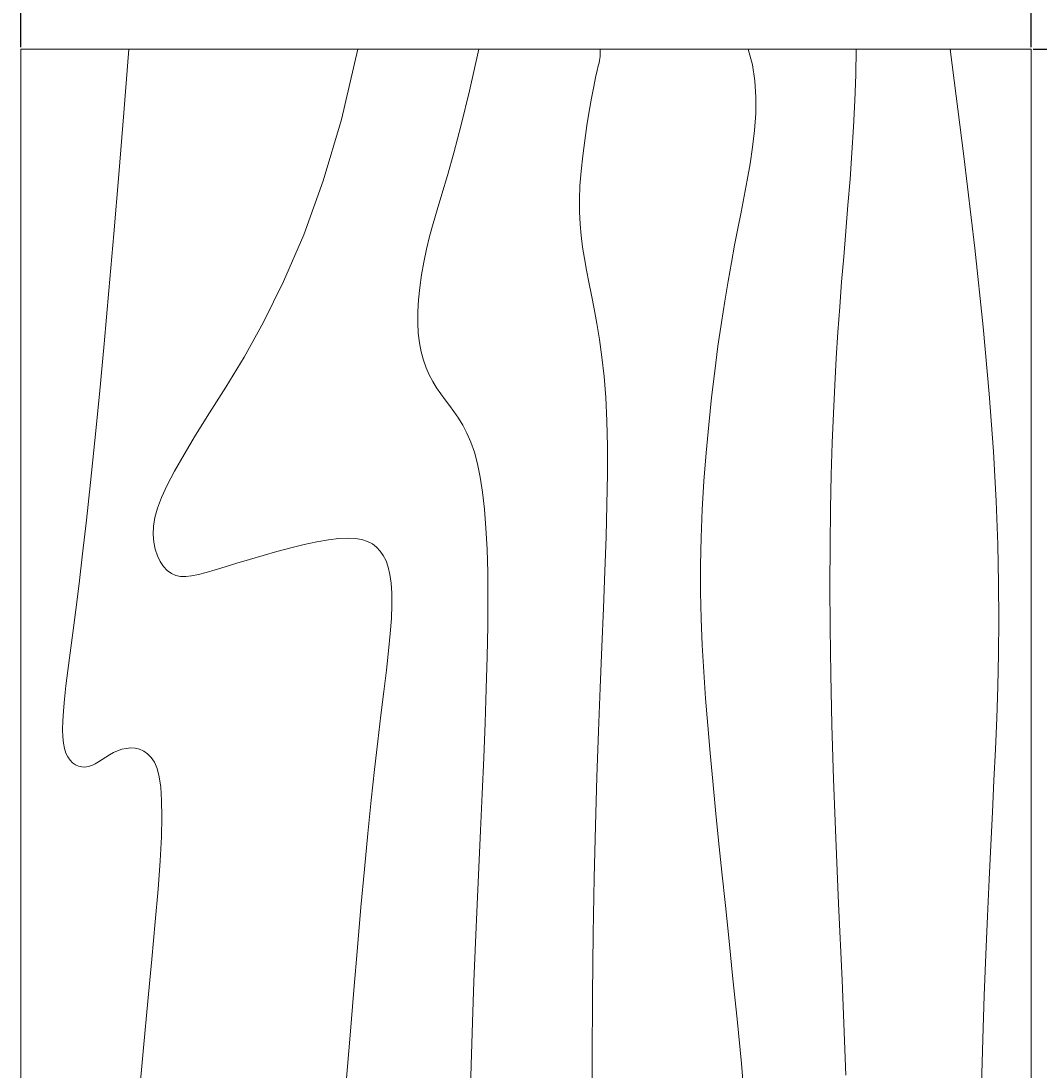
# Model space of a CAD drawing. Units: inches. Extents: x -105 to 1196, y -792 to 119.
# Tile 13 of 23: x 232 to 262, y -349 to -318. Entities that reach past the tile are written whole.
import ezdxf

# ---------------------------------------------------------------- set-up
doc = ezdxf.new("R2010")
doc.units = ezdxf.units.IN
doc.header["$MEASUREMENT"] = 0
doc.layers.add('A-ANNO-DIMS', color=2, linetype='Continuous', lineweight=18)
doc.layers.add('A-FURN', color=8, linetype='Continuous', lineweight=18)
doc.styles.get("Standard").update_dxf_attribs({"font": 'arial.ttf'})
doc.dimstyles.get("Standard").update_dxf_attribs({"dimtxt": 0.18, "dimasz": 0.18, "dimexe": 0.18, "dimexo": 0.0625, "dimgap": 0.09, "dimtad": 0, "dimtih": 1, "dimtoh": 1, "dimdec": 1, "dimzin": 0, "dimdsep": 46, "dimlunit": 4, "dimtxsty": 'Standard', "dimcen": 0.09, "dimadec": 0, "dimazin": 0, "dimtfac": 1, "dimtdec": 1, "dimtofl": 0, "dimtmove": 0, "dimatfit": 3, "dimfxl": 1, "dimtolj": 1, "dimtzin": 0, "dimarcsym": 0})

# ---------------------------------------------------------------- blocks, each defined once
blk = doc.blocks.new('Table - Rectangular Woodgrain 60 x 30 in.')
for p, q in [((60, 0), (0, 0)), ((60, -30), (60, 0)), ((0, -30), (60, -30))]:
    blk.add_line(p, q)
for points in [[(28.8172, -3.4958), (30.3437, -3.636), (31.7291, -3.7667), (32.9756, -3.8849), (34.0849, -3.9875), (35.059, -4.0714), (35.9, -4.1334), (36.6114, -4.1711), (37.2041, -4.1854), (37.6906, -4.1779), (38.0833, -4.15), (38.3948, -4.1034), (38.6375, -4.0396), (38.8239, -3.9602), (38.9666, -3.8667), (39.0764, -3.7608), (39.1573, -3.6448), (39.2116, -3.521), (39.2416, -3.3917), (39.2498, -3.2593), (39.2385, -3.1261), (39.21, -2.9944), (39.1666, -2.8667), (39.111, -2.7447), (39.0468, -2.6281), (38.978, -2.5163), (38.9083, -2.4083), (38.8418, -2.3035), (38.7823, -2.201), (38.7337, -2.1001), (38.7, -2), (38.6844, -1.9003), (38.6875, -1.8021), (38.7094, -1.707), (38.75, -1.6167), (38.8094, -1.5326), (38.8875, -1.4563), (38.9844, -1.3893), (39.1, -1.3333), (39.2351, -1.2896), (39.3937, -1.2583), (39.5804, -1.2396), (39.8, -1.2333), (40.057, -1.2396), (40.3562, -1.2583), (40.7023, -1.2896), (41.1, -1.3333), (41.5547, -1.3895), (42.0755, -1.4573), (42.6721, -1.5361), (43.3542, -1.625), (44.1316, -1.7233), (45.014, -1.8302), (46.0114, -1.9449), (47.1333, -2.0667), (48.3862, -2.1947), (49.7625, -2.3281), (51.2513, -2.4663), (52.8416, -2.6083), (54.5226, -2.7535), (56.2833, -2.9011), (58.1127, -3.0501), (60, -3.2)], [(29.3241, -9.6553), (30.7203, -9.7719), (32.0532, -9.8837), (33.3208, -9.9917), (34.5213, -10.0965), (35.6526, -10.199), (36.7128, -10.2999), (37.7, -10.4), (38.6129, -10.4996), (39.4531, -10.5969), (40.223, -10.6895), (40.925, -10.775), (41.5613, -10.8512), (42.1344, -10.9156), (42.6465, -10.966), (43.1, -11), (43.4976, -11.0158), (43.8437, -11.0136), (44.143, -10.9942), (44.4, -10.9583), (44.6195, -10.9069), (44.8062, -10.8406), (44.9648, -10.7603), (45.1, -10.6667), (45.2155, -10.5598), (45.3114, -10.4365), (45.3871, -10.2929), (45.4416, -10.125), (45.4743, -9.929), (45.4844, -9.7011), (45.4709, -9.4371), (45.4333, -9.1333), (45.3716, -8.7883), (45.2896, -8.4104), (45.1919, -8.0107), (45.0833, -7.6), (44.9685, -7.1893), (44.8521, -6.7896), (44.7388, -6.4117), (44.6333, -6.0667), (44.54, -5.7628), (44.4614, -5.4979), (44.4001, -5.2675), (44.3583, -5.0667), (44.3384, -4.8909), (44.3427, -4.7354), (44.3736, -4.5956), (44.4333, -4.4667), (44.5236, -4.3453), (44.6427, -4.2333), (44.7884, -4.1339), (44.9583, -4.05), (45.1501, -3.9849), (45.3614, -3.9417), (45.59, -3.9234), (45.8333, -3.9333), (46.0915, -3.9749), (46.3734, -4.0531), (46.6906, -4.1736), (47.0542, -4.3417), (47.4756, -4.5629), (47.9661, -4.8427), (48.5372, -5.1866), (49.2, -5.6), (49.9676, -6.0844), (50.8594, -6.625), (51.8965, -7.2031), (53.1, -7.8), (54.491, -8.3969), (56.0906, -8.975), (57.9199, -9.5156), (60, -10)], [(28.4531, -13.3281), (29.8256, -13.3663), (31.1083, -13.4083), (32.3191, -13.4535), (33.476, -13.501), (34.597, -13.5501), (35.7, -13.6), (36.7984, -13.6497), (37.8875, -13.6979), (38.9578, -13.743), (40, -13.7833), (41.0047, -13.8174), (41.9625, -13.8438), (42.864, -13.8607), (43.7, -13.8667), (44.4631, -13.8604), (45.1552, -13.8417), (45.7801, -13.8104), (46.3416, -13.7667), (46.8439, -13.7104), (47.2906, -13.6417), (47.6858, -13.5604), (48.0333, -13.4667), (48.3375, -13.3608), (48.6042, -13.2448), (48.8396, -13.121), (49.05, -12.9917), (49.2417, -12.8593), (49.4208, -12.7261), (49.5937, -12.5944), (49.7667, -12.4667), (49.9452, -12.3451), (50.1323, -12.2313), (50.3303, -12.1268), (50.5416, -12.0333), (50.7686, -11.9524), (51.0135, -11.8854), (51.2788, -11.8341), (51.5666, -11.8), (51.8785, -11.7843), (52.2116, -11.7865), (52.562, -11.8059), (52.926, -11.8417), (53.2998, -11.8931), (53.6795, -11.9594), (54.0614, -12.0397), (54.4416, -12.1333), (54.8223, -12.2401), (55.2293, -12.3625), (55.6942, -12.5037), (56.2489, -12.6667), (56.9251, -12.8547), (57.7545, -13.0708), (58.7689, -13.3182), (60, -13.6)], [(27.9, -16.9667), (29.9928, -16.9617), (31.9302, -16.9703), (33.7254, -16.9907), (35.3917, -17.0208), (36.9423, -17.0588), (38.3906, -17.1026), (39.7499, -17.1503), (41.0333, -17.2), (42.2519, -17.2496), (43.4073, -17.2969), (44.4986, -17.3395), (45.525, -17.375), (46.4858, -17.4012), (47.3802, -17.4156), (48.2074, -17.416), (48.9667, -17.4), (49.6583, -17.3662), (50.2872, -17.3167), (50.8595, -17.2547), (51.3812, -17.1833), (51.8584, -17.1057), (52.2971, -17.025), (52.7034, -16.9443), (53.0833, -16.8667), (53.443, -16.7951), (53.789, -16.7313), (54.128, -16.6768), (54.4666, -16.6334), (54.8115, -16.6024), (55.1693, -16.5854), (55.5465, -16.5841), (55.95, -16.6), (56.3828, -16.6337), (56.8346, -16.6823), (57.2915, -16.7418), (57.7396, -16.8084), (58.165, -16.878), (58.5539, -16.9469), (58.8924, -17.0111), (59.1666, -17.0667), (59.3679, -17.1107), (59.5078, -17.1438), (59.6032, -17.1675), (59.6708, -17.1833), (59.7275, -17.193), (59.7901, -17.1979), (59.8753, -17.1998), (60, -17.2)], [(28.2656, -21.5281), (29.884, -21.3947), (31.2, -21.2667), (32.3967, -21.1448), (33.5172, -21.0292), (34.5697, -20.9198), (35.5625, -20.8167), (36.5037, -20.7198), (37.4015, -20.6292), (38.2642, -20.5448), (39.1, -20.4667), (39.9164, -20.3951), (40.7187, -20.3313), (41.5117, -20.2768), (42.3, -20.2333), (43.0883, -20.2024), (43.8812, -20.1854), (44.6836, -20.1841), (45.5, -20.2), (46.3328, -20.234), (47.1747, -20.2844), (48.0163, -20.3488), (48.8479, -20.425), (49.66, -20.5106), (50.4429, -20.6031), (51.1872, -20.7004), (51.8833, -20.8), (52.5246, -20.8999), (53.1166, -20.9995), (53.6681, -21.0983), (54.1875, -21.1958), (54.6834, -21.2919), (55.1646, -21.3859), (55.6394, -21.4777), (56.1167, -21.5667), (56.6028, -21.6515), (57.0961, -21.7266), (57.5929, -21.7852), (58.0896, -21.8208), (58.5823, -21.8268), (59.0674, -21.7964), (59.5412, -21.723), (60, -21.6)], [(29.529, -24.4988), (32.3578, -24.3844), (34.6359, -24.284), (36.5667, -24.2), (38.3213, -24.1341), (39.9417, -24.0854), (41.437, -24.0523), (42.8167, -24.0333), (44.0901, -24.0268), (45.2667, -24.0313), (46.3557, -24.0451), (47.3667, -24.0667), (48.309, -24.0947), (49.1928, -24.1287), (50.0284, -24.168), (50.826, -24.2125), (51.5959, -24.2617), (52.3483, -24.3151), (53.0935, -24.3725), (53.8417, -24.4334), (54.6009, -24.497), (55.3699, -24.561), (56.1454, -24.6226), (56.9239, -24.6792), (57.7021, -24.7279), (58.4764, -24.7662), (59.2435, -24.7911), (60, -24.8)], [(29.2276, -28.5281), (30.6033, -28.5663), (31.8958, -28.6084), (33.1118, -28.6535), (34.2578, -28.7011), (35.3405, -28.7501), (36.3666, -28.8), (37.3443, -28.8497), (38.288, -28.8974), (39.2137, -28.9412), (40.1375, -28.9792), (41.0753, -29.0093), (42.0432, -29.0297), (43.0572, -29.0384), (44.1333, -29.0333), (45.2936, -29.0114), (46.5843, -28.9641), (48.0579, -28.8816), (49.7666, -28.7542), (51.7629, -28.5721), (54.0989, -28.3255), (56.8272, -28.0048), (60, -27.6)]]:
    blk.add_lwpolyline(points)
blk = doc.blocks.new('*D83')
at = {"layer": 'A-ANNO-DIMS', "color": 0, "lineweight": -2, "transparency": 16777216}
for p, q in [((261.878, -318.695), (270.995, -318.695)), ((270.815, -318.875), (270.815, -348.512)), ((270.815, -378.515), (270.815, -348.878)), ((261.878, -378.695), (270.995, -378.695))]:
    blk.add_line(p, q, dxfattribs=at)
at = {"layer": 'A-ANNO-DIMS', "color": 0, "transparency": 16777216}
for points in [[(270.785, -318.875), (270.845, -318.875), (270.815, -318.695)], [(270.785, -378.515), (270.845, -378.515), (270.815, -378.695)]]:
    blk.add_solid(points, dxfattribs=at)
at = {"layer": 'Defpoints', "color": 0, "transparency": 16777216}
for p in [(261.815, -318.695), (270.815, -318.695), (261.815, -378.695)]:
    blk.add_point(p, dxfattribs=at)
at = {"layer": 'A-ANNO-DIMS', "color": 0, "transparency": 16777216, "insert": (270.815, -348.695), "char_height": 0.18, "attachment_point": 5}
blk.add_mtext('\\A1;CENTRE TABLE 5\'-0"', dxfattribs=at)
blk = doc.blocks.new('*D84')
at = {"layer": 'A-ANNO-DIMS', "color": 0, "lineweight": -2, "transparency": 16777216}
for p, q in [((231.815, -318.633), (231.815, -309.515)), ((261.815, -318.633), (261.815, -309.515)), ((231.995, -309.695), (246.484, -309.695)), ((261.635, -309.695), (247.146, -309.695))]:
    blk.add_line(p, q, dxfattribs=at)
at = {"layer": 'A-ANNO-DIMS', "color": 0, "transparency": 16777216}
for points in [[(231.995, -309.665), (231.995, -309.725), (231.815, -309.695)], [(261.635, -309.665), (261.635, -309.725), (261.815, -309.695)]]:
    blk.add_solid(points, dxfattribs=at)
at = {"layer": 'Defpoints', "color": 0, "transparency": 16777216}
for p in [(231.815, -309.695), (231.815, -318.695), (261.815, -318.695)]:
    blk.add_point(p, dxfattribs=at)
at = {"layer": 'A-ANNO-DIMS', "color": 0, "transparency": 16777216, "insert": (246.815, -309.695), "char_height": 0.18, "attachment_point": 5}
blk.add_mtext('\\A1;2\'-6"', dxfattribs=at)

msp = doc.modelspace()

# ---------------------------------------------------------------- block references
at = {"layer": 'A-FURN', "rotation": 90}
msp.add_blockref('Table - Rectangular Woodgrain 60 x 30 in.', (231.815, -378.695), dxfattribs=at)

# ---------------------------------------------------------------- dimensions: what is measured, and where the dimension line sits
at = {"layer": 'A-ANNO-DIMS'}
dim = msp.add_linear_dim(base=(231.815, -309.695), p1=(261.815, -318.695), p2=(231.815, -318.695), angle=180, dimstyle='Standard', override={"dimdec": 1, "dimlfac": 1, "dimrnd": 0, "dimzin": 1, "dimdsep": 46, "dimlunit": 4, "dimfrac": 2}, dxfattribs=at)
dim.commit()
dim.dimension.update_dxf_attribs({"geometry": '*D84', "text_midpoint": (246.815, -309.695)})
dim = msp.add_linear_dim(base=(270.815, -318.695), p1=(261.815, -378.695), p2=(261.815, -318.695), angle=90, text='CENTRE TABLE <>', dimstyle='Standard', override={"dimdec": 1, "dimlfac": 1, "dimrnd": 0, "dimzin": 1, "dimdsep": 46, "dimlunit": 4, "dimfrac": 2}, dxfattribs=at)
dim.commit()
dim.dimension.update_dxf_attribs({"geometry": '*D83', "text_midpoint": (270.815, -348.695)})

doc.saveas('drawing.dxf')
